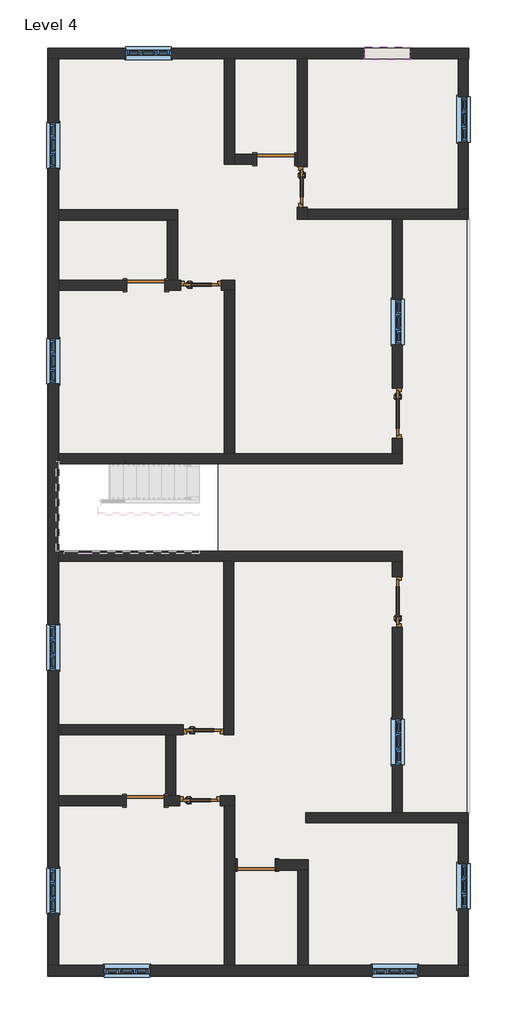
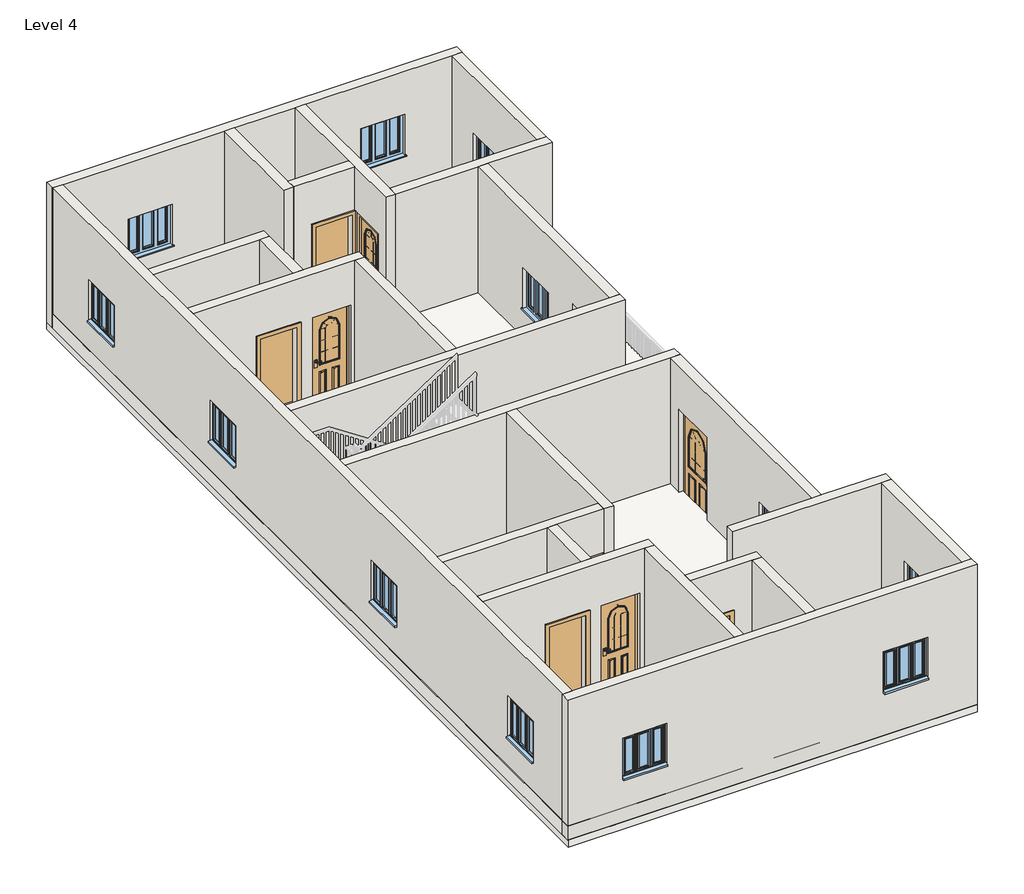
# One storey, part 1 of 3: 25 walls, 12 windows, 10 doors, 1 roof, 1 slab.
"""IFC4 building model written with IfcOpenShell, lengths in millimetres."""

from ifc_helpers import new_model, si_unit, frame, origin, place, context, project, spatial, polyline, outline, extrude, faceted_brep, transform, mapped, element, save
from components import doors_extsgl_w_glazing_bars_arched_1010x2110mm_bccdb1b2, doors_extsgl_w_glazing_bars_arched_1010x2110mm_5c897e1f, doors_extsgl_w_glazing_bars_arched_810x2110mm_57ea6d9e, doors_extsgl_w_glazing_bars_arched_810x2110mm_84a0a083, door_fadea3f2, windows_tpl_w_glazing_bars_910x910mm_9d987a72

model = new_model("IFC4")

# Units and contexts
model_context = context("Model", 3, world=origin())
ifc_project = project(units=[si_unit("LENGTHUNIT", "METRE", prefix="MILLI")], contexts=[model_context])

# Site, building, storey
site = spatial("IfcSite", under=ifc_project)
building = spatial("IfcBuilding", under=site)
storey = spatial("IfcBuildingStorey", under=building, Name="Level 4", Elevation=9144.0)

# Doors
placement = place(None, origin())
doors_extsgl_w_glazing_bars_arched_1010x2110mm_shape = doors_extsgl_w_glazing_bars_arched_1010x2110mm_bccdb1b2(model_context)
element("IfcDoor", 1, ObjectType="Doors_ExtSgl_w-Glazing_Bars_Arched : 1010x2110mm", at=placement, inside=storey, context=model_context, shape_type="MappedRepresentation", body=[
    mapped(doors_extsgl_w_glazing_bars_arched_1010x2110mm_shape, transform((1850.5605895, 2208.5797121, 9144.0), x_axis=(0.0, -1.0, 0.0), y_axis=(1.0, 0.0, 0.0), z_axis=(0.0, 0.0, 1.0))),
])
doors_extsgl_w_glazing_bars_arched_1010x2110mm_2_shape = doors_extsgl_w_glazing_bars_arched_1010x2110mm_5c897e1f(model_context)
element("IfcDoor", 2, ObjectType="Doors_ExtSgl_w-Glazing_Bars_Arched : 1010x2110mm", at=placement, inside=storey, context=model_context, shape_type="MappedRepresentation", body=[
    mapped(doors_extsgl_w_glazing_bars_arched_1010x2110mm_2_shape, transform((1850.5605895, -1576.0202879, 9144.0), x_axis=(0.0, 1.0, 0.0), y_axis=(-1.0, 0.0, 0.0), z_axis=(0.0, 0.0, 1.0))),
])
doors_extsgl_w_glazing_bars_arched_810x2110mm_shape = doors_extsgl_w_glazing_bars_arched_810x2110mm_57ea6d9e(model_context)
element("IfcDoor", 3, ObjectType="Doors_ExtSgl_w-Glazing_Bars_Arched : 810x2110mm", at=placement, inside=storey, context=model_context, shape_type="MappedRepresentation", body=[
    mapped(doors_extsgl_w_glazing_bars_arched_810x2110mm_shape, transform((-2086.4394105, 4773.9797121, 9144.0), x_axis=(1.0, 0.0, 0.0), y_axis=(0.0, 1.0, 0.0), z_axis=(0.0, 0.0, 1.0))),
])
element("IfcDoor", 4, ObjectType="Doors_ExtSgl_w-Glazing_Bars_Arched : 810x2110mm", at=placement, inside=storey, context=model_context, shape_type="MappedRepresentation", body=[
    mapped(doors_extsgl_w_glazing_bars_arched_810x2110mm_shape, transform((-2105.4894105, -5563.8202879, 9144.0), x_axis=(1.0, 0.0, 0.0), y_axis=(0.0, 1.0, 0.0), z_axis=(0.0, 0.0, 1.0))),
])
doors_extsgl_w_glazing_bars_arched_810x2110mm_2_shape = doors_extsgl_w_glazing_bars_arched_810x2110mm_84a0a083(model_context)
element("IfcDoor", 5, ObjectType="Doors_ExtSgl_w-Glazing_Bars_Arched : 810x2110mm", at=placement, inside=storey, context=model_context, shape_type="MappedRepresentation", body=[
    mapped(doors_extsgl_w_glazing_bars_arched_810x2110mm_2_shape, transform((-2035.6394105, -4141.4202879, 9144.0), x_axis=(1.0, 0.0, 0.0), y_axis=(0.0, 1.0, 0.0), z_axis=(0.0, 0.0, 1.0))),
])
element("IfcDoor", 6, ObjectType="Doors_ExtSgl_w-Glazing_Bars_Arched : 810x2110mm", at=placement, inside=storey, context=model_context, shape_type="MappedRepresentation", body=[
    mapped(doors_extsgl_w_glazing_bars_arched_810x2110mm_2_shape, transform((-54.4394105, 6748.5640518, 9144.0), x_axis=(0.0, -1.0, 0.0), y_axis=(1.0, 0.0, 0.0), z_axis=(0.0, 0.0, 1.0))),
])
door_shape = door_fadea3f2(model_context)
element("IfcDoor", 7, ObjectType="Single-Flush : 30\" x 80\"", at=placement, inside=storey, context=model_context, shape_type="MappedRepresentation", body=[
    mapped(door_shape, transform((-3204.0394105, -5563.8202879, 9144.0), x_axis=(1.0, 0.0, 0.0), y_axis=(0.0, 1.0, 0.0), z_axis=(0.0, 0.0, 1.0))),
])
element("IfcDoor", 8, ObjectType="Single-Flush : 30\" x 80\"", at=placement, inside=storey, context=model_context, shape_type="MappedRepresentation", body=[
    mapped(door_shape, transform((-981.5394105, -6850.9128362, 9144.0), x_axis=(-1.0, 0.0, 0.0), y_axis=(0.0, -1.0, 0.0), z_axis=(0.0, 0.0, 1.0))),
])
element("IfcDoor", 9, ObjectType="Single-Flush : 30\" x 80\"", at=placement, inside=storey, context=model_context, shape_type="MappedRepresentation", body=[
    mapped(door_shape, transform((-3191.3394105, 4773.9797121, 9144.0), x_axis=(1.0, 0.0, 0.0), y_axis=(0.0, 1.0, 0.0), z_axis=(0.0, 0.0, 1.0))),
])
element("IfcDoor", 10, ObjectType="Single-Flush : 30\" x 80\"", at=placement, inside=storey, context=model_context, shape_type="MappedRepresentation", body=[
    mapped(door_shape, transform((-587.8394105, 7301.2797121, 9144.0), x_axis=(1.0, 0.0, 0.0), y_axis=(0.0, 1.0, 0.0), z_axis=(0.0, 0.0, 1.0))),
])

# Roof
element("IfcRoof", 11, ObjectType="Generic - 12\"", at=placement, inside=storey, context=model_context, shape_type="SweptSolid", body=[
    extrude(outline(polyline([(3272.9605895, 9523.7797121), (3272.9605895, -9069.0202879), (-5159.8394105, -9069.0202879), (-5159.8394105, 9523.7797121), (3272.9605895, 9523.7797121)]), holes=[polyline([(-1756.1922756, 1192.5797121), (-4943.9394105, 1192.5797121), (-4943.9394105, -560.0202879), (-1756.1922756, -560.0202879), (-1756.1922756, 1192.5797121)])]), frame((0.0, 0.0, 9144.0), z_axis=(0.0, 0.0, 1.0), x_axis=(1.0, 0.0, 0.0)), (0.0, 0.0, 1.0), 304.8),
])

# Slab
element("IfcSlab", 12, ObjectType="Generic - 12\"", at=placement, inside=storey, context=model_context, shape_type="SweptSolid", body=[
    extrude(outline(polyline([(3272.9605895, 9523.7797121), (3272.9605895, -9081.7202879), (-5159.8394105, -9081.7202879), (-5159.8394105, 9523.7797121), (3272.9605895, 9523.7797121)]), holes=[polyline([(-1756.1922756, 1192.5797121), (-4943.9394105, 1192.5797121), (-4943.9394105, -560.0202879), (-1756.1922756, -560.0202879), (-1756.1922756, 1192.5797121)])]), frame((0.0, 0.0, 8991.6), z_axis=(0.0, 0.0, 1.0), x_axis=(1.0, 0.0, 0.0)), (0.0, 0.0, 1.0), 152.4),
])

# Walls
element("IfcWall", 13, ObjectType="Generic - 4.5\" p", at=placement, inside=storey, context=model_context, shape_type="Brep", body=[
    faceted_brep([(-2810.3394105, 4672.3797121, 11176.0), (-2810.3394105, 4672.3797121, 9144.0), (-2491.4394105, 4672.3797121, 9144.0), (-2491.4394105, 4672.3797121, 11254.0), (-1681.4394105, 4672.3797121, 11254.0), (-1681.4394105, 4672.3797121, 9144.0), (-1616.5394105, 4672.3797121, 9144.0), (-1413.3394105, 4672.3797121, 9144.0), (-1413.3394105, 4672.3797121, 12192.0), (-1616.5394105, 4672.3797121, 12192.0), (-4943.9394105, 4672.3797121, 12192.0), (-4943.9394105, 4672.3797121, 9144.0), (-3572.3394105, 4672.3797121, 9144.0), (-3572.3394105, 4672.3797121, 11176.0), (-2491.4394105, 4875.5797121, 9144.0), (-2556.3394105, 4875.5797121, 9144.0), (-2759.5394105, 4875.5797121, 9144.0), (-2810.3394105, 4875.5797121, 9144.0), (-2810.3394105, 4875.5797121, 11176.0), (-3572.3394105, 4875.5797121, 11176.0), (-3572.3394105, 4875.5797121, 9144.0), (-4943.9394105, 4875.5797121, 9144.0), (-4943.9394105, 4875.5797121, 12192.0), (-2759.5394105, 4875.5797121, 12192.0), (-2556.3394105, 4875.5797121, 12192.0), (-1413.3394105, 4875.5797121, 12192.0), (-1413.3394105, 4875.5797121, 9144.0), (-1681.4394105, 4875.5797121, 9144.0), (-1681.4394105, 4875.5797121, 11254.0), (-2491.4394105, 4875.5797121, 11254.0)], [[[0, 1, 2, 3, 4, 5, 6, 7, 8, 9, 10, 11, 12, 13]], [[14, 15, 16, 17, 18, 19, 20, 21, 22, 23, 24, 25, 26, 27, 28, 29]], [[7, 6, 5, 27, 26]], [[12, 11, 21, 20]], [[2, 1, 17, 16, 15, 14]], [[10, 9, 8, 25, 24, 23, 22]], [[11, 10, 22, 21]], [[8, 7, 26, 25]], [[14, 29, 3, 2]], [[28, 27, 5, 4]], [[29, 28, 4, 3]], [[18, 17, 1, 0]], [[19, 18, 0, 13]], [[20, 19, 13, 12]]]),
])
element("IfcWall", 14, ObjectType="Generic - 4.5\" p", at=placement, inside=storey, context=model_context, shape_type="SweptSolid", body=[
    extrude(outline(polyline([(-1616.5394105, 1395.7797121), (-1616.5394105, 4672.3797121), (-1413.3394105, 4672.3797121), (-1413.3394105, 1395.7797121), (-1616.5394105, 1395.7797121)])), frame((0.0, 0.0, 9144.0), z_axis=(0.0, 0.0, 1.0), x_axis=(1.0, 0.0, 0.0)), (0.0, 0.0, 1.0), 3048.0),
])
element("IfcWall", 15, ObjectType="Generic - 4.5\" p", at=placement, inside=storey, context=model_context, shape_type="Brep", body=[
    faceted_brep([(-4943.9394105, 6082.1542467, 9144.0), (-2759.5394105, 6082.1542467, 9144.0), (-2556.3394105, 6082.1542467, 9144.0), (-2556.3394105, 6082.1542467, 12192.0), (-2759.5394105, 6082.1542467, 12192.0), (-4943.9394105, 6082.1542467, 12192.0), (-4943.9394105, 6285.3542467, 9144.0), (-4943.9394105, 6285.3542467, 12192.0), (-2556.3394105, 6285.3542467, 12192.0), (-2556.3394105, 6285.3542467, 9144.0)], [[[0, 1, 2, 3, 4, 5]], [[6, 7, 8, 9]], [[2, 1, 0, 6, 9]], [[5, 4, 3, 8, 7]], [[0, 5, 7, 6]], [[3, 2, 9, 8]]]),
])
element("IfcWall", 16, ObjectType="Generic - 4.5\" p", at=placement, inside=storey, context=model_context, shape_type="SweptSolid", body=[
    extrude(outline(polyline([(-2759.5394105, 4875.5797121), (-2759.5394105, 6082.1542467), (-2556.3394105, 6082.1542467), (-2556.3394105, 4875.5797121), (-2759.5394105, 4875.5797121)])), frame((0.0, 0.0, 9144.0), z_axis=(0.0, 0.0, 1.0), x_axis=(1.0, 0.0, 0.0)), (0.0, 0.0, 1.0), 3048.0),
])
element("IfcWall", 17, ObjectType="Generic - 4.5\" p", at=placement, inside=storey, context=model_context, shape_type="Brep", body=[
    faceted_brep([(-1616.5394105, 9320.5797121, 9144.0), (-1616.5394105, 7199.6797121, 9144.0), (-1616.5394105, 7199.6797121, 12192.0), (-1616.5394105, 9320.5797121, 12192.0), (-1413.3394105, 9320.5797121, 9144.0), (-1413.3394105, 9320.5797121, 12192.0), (-1413.3394105, 7402.8797121, 12192.0), (-1413.3394105, 7199.6797121, 12192.0), (-1413.3394105, 7199.6797121, 9144.0), (-1413.3394105, 7402.8797121, 9144.0)], [[[0, 1, 2, 3]], [[4, 5, 6, 7, 8, 9]], [[1, 0, 4, 9, 8]], [[3, 2, 7, 6, 5]], [[0, 3, 5, 4]], [[2, 1, 8, 7]]]),
])
element("IfcWall", 18, ObjectType="Generic - 4.5\" p", at=placement, inside=storey, context=model_context, shape_type="SweptSolid", body=[
    extrude(outline(polyline([(11176.0, -206.8394105), (9144.0, -206.8394105), (9144.0, -156.0394105), (12192.0, -156.0394105), (12192.0, -1413.3394105), (9144.0, -1413.3394105), (9144.0, -968.8394105), (11176.0, -968.8394105), (11176.0, -206.8394105)])), frame((0.0, 7199.6797121, 0.0), z_axis=(0.0, 1.0, 0.0), x_axis=(0.0, 0.0, 1.0)), (0.0, 0.0, 1.0), 203.2),
])
element("IfcWall", 19, ObjectType="Generic - 4.5\" p", at=placement, inside=storey, context=model_context, shape_type="Brep", body=[
    faceted_brep([(-156.0394105, 6343.5640518, 11254.0), (-156.0394105, 6343.5640518, 9144.0), (-156.0394105, 6094.2483916, 9144.0), (-156.0394105, 6094.2483916, 12192.0), (-156.0394105, 7199.6797121, 12192.0), (-156.0394105, 7402.8797121, 12192.0), (-156.0394105, 9320.5797121, 12192.0), (-156.0394105, 9320.5797121, 9144.0), (-156.0394105, 7402.8797121, 9144.0), (-156.0394105, 7199.6797121, 9144.0), (-156.0394105, 7153.5640518, 9144.0), (-156.0394105, 7153.5640518, 11254.0), (47.1605895, 6094.2483916, 9144.0), (47.1605895, 6297.4483916, 9144.0), (47.1605895, 6343.5640518, 9144.0), (47.1605895, 6343.5640518, 11254.0), (47.1605895, 7153.5640518, 11254.0), (47.1605895, 7153.5640518, 9144.0), (47.1605895, 9320.5797121, 9144.0), (47.1605895, 9320.5797121, 12192.0), (47.1605895, 6297.4483916, 12192.0), (47.1605895, 6094.2483916, 12192.0)], [[[0, 1, 2, 3, 4, 5, 6, 7, 8, 9, 10, 11]], [[12, 13, 14, 15, 16, 17, 18, 19, 20, 21]], [[2, 1, 14, 13, 12]], [[10, 9, 8, 7, 18, 17]], [[6, 5, 4, 3, 21, 20, 19]], [[7, 6, 19, 18]], [[3, 2, 12, 21]], [[17, 16, 11, 10]], [[15, 14, 1, 0]], [[16, 15, 0, 11]]]),
])
element("IfcWall", 20, ObjectType="Generic - 4.5\" p", at=placement, inside=storey, context=model_context, shape_type="Brep", body=[
    faceted_brep([(47.1605895, 6094.2483916, 9144.0), (1748.9605895, 6094.2483916, 9144.0), (1952.1605895, 6094.2483916, 9144.0), (3272.9605895, 6094.2483916, 9144.0), (3272.9605895, 6094.2483916, 12192.0), (1952.1605895, 6094.2483916, 12192.0), (1748.9605895, 6094.2483916, 12192.0), (47.1605895, 6094.2483916, 12192.0), (47.1605895, 6297.4483916, 9144.0), (47.1605895, 6297.4483916, 12192.0), (3069.7605895, 6297.4483916, 12192.0), (3272.9605895, 6297.4483916, 12192.0), (3272.9605895, 6297.4483916, 9144.0), (3069.7605895, 6297.4483916, 9144.0)], [[[0, 1, 2, 3, 4, 5, 6, 7]], [[8, 9, 10, 11, 12, 13]], [[3, 2, 1, 0, 8, 13, 12]], [[7, 6, 5, 4, 11, 10, 9]], [[0, 7, 9, 8]], [[4, 3, 12, 11]]]),
])
element("IfcWall", 21, ObjectType="Generic - 4.5\" p", at=placement, inside=storey, context=model_context, shape_type="Brep", body=[
    faceted_brep([(-4943.9394105, 1192.5797121, 9144.0), (1952.1605895, 1192.5797121, 9144.0), (1952.1605895, 1192.5797121, 12192.0), (-4943.9394105, 1192.5797121, 12192.0), (-4943.9394105, 1395.7797121, 9144.0), (-4943.9394105, 1395.7797121, 12192.0), (-1616.5394105, 1395.7797121, 12192.0), (-1413.3394105, 1395.7797121, 12192.0), (1748.9605895, 1395.7797121, 12192.0), (1952.1605895, 1395.7797121, 12192.0), (1952.1605895, 1395.7797121, 9144.0), (1748.9605895, 1395.7797121, 9144.0), (-1413.3394105, 1395.7797121, 9144.0), (-1616.5394105, 1395.7797121, 9144.0)], [[[0, 1, 2, 3]], [[4, 5, 6, 7, 8, 9, 10, 11, 12, 13]], [[1, 0, 4, 13, 12, 11, 10]], [[3, 2, 9, 8, 7, 6, 5]], [[0, 3, 5, 4]], [[2, 1, 10, 9]]]),
])
element("IfcWall", 22, ObjectType="Generic - 4.5\" p", at=placement, inside=storey, context=model_context, shape_type="Brep", body=[
    faceted_brep([(-4943.9394105, -763.2202879, 9144.0), (-1629.2394105, -763.2202879, 9144.0), (-1426.0394105, -763.2202879, 9144.0), (1748.9605895, -763.2202879, 9144.0), (1952.1605895, -763.2202879, 9144.0), (1952.1605895, -763.2202879, 12192.0), (1748.9605895, -763.2202879, 12192.0), (-1426.0394105, -763.2202879, 12192.0), (-1629.2394105, -763.2202879, 12192.0), (-4943.9394105, -763.2202879, 12192.0), (-4943.9394105, -560.0202879, 9144.0), (-4943.9394105, -560.0202879, 12192.0), (1952.1605895, -560.0202879, 12192.0), (1952.1605895, -560.0202879, 9144.0)], [[[0, 1, 2, 3, 4, 5, 6, 7, 8, 9]], [[10, 11, 12, 13]], [[4, 3, 2, 1, 0, 10, 13]], [[9, 8, 7, 6, 5, 12, 11]], [[0, 9, 11, 10]], [[5, 4, 13, 12]]]),
])
element("IfcWall", 23, ObjectType="Generic - 4.5\" p", at=placement, inside=storey, context=model_context, shape_type="Brep", body=[
    faceted_brep([(-1629.2394105, -763.2202879, 9144.0), (-1629.2394105, -4039.8202879, 9144.0), (-1629.2394105, -4243.0202879, 9144.0), (-1629.2394105, -4243.0202879, 12192.0), (-1629.2394105, -4039.8202879, 12192.0), (-1629.2394105, -763.2202879, 12192.0), (-1426.0394105, -763.2202879, 9144.0), (-1426.0394105, -763.2202879, 12192.0), (-1426.0394105, -4243.0202879, 12192.0), (-1426.0394105, -4243.0202879, 9144.0)], [[[0, 1, 2, 3, 4, 5]], [[6, 7, 8, 9]], [[2, 1, 0, 6, 9]], [[5, 4, 3, 8, 7]], [[0, 5, 7, 6]], [[3, 2, 9, 8]]]),
])
element("IfcWall", 24, ObjectType="Generic - 4.5\" p", at=placement, inside=storey, context=model_context, shape_type="Brep", body=[
    faceted_brep([(-1630.6394105, -4243.0202879, 11254.0), (-1630.6394105, -4243.0202879, 9144.0), (-1629.2394105, -4243.0202879, 9144.0), (-1629.2394105, -4243.0202879, 12192.0), (-2594.4394105, -4243.0202879, 12192.0), (-2797.6394105, -4243.0202879, 12192.0), (-4943.9394105, -4243.0202879, 12192.0), (-4943.9394105, -4243.0202879, 9144.0), (-2797.6394105, -4243.0202879, 9144.0), (-2594.4394105, -4243.0202879, 9144.0), (-2440.6394105, -4243.0202879, 9144.0), (-2440.6394105, -4243.0202879, 11254.0), (-1629.2394105, -4039.8202879, 9144.0), (-1630.6394105, -4039.8202879, 9144.0), (-1630.6394105, -4039.8202879, 11254.0), (-2440.6394105, -4039.8202879, 11254.0), (-2440.6394105, -4039.8202879, 9144.0), (-4943.9394105, -4039.8202879, 9144.0), (-4943.9394105, -4039.8202879, 12192.0), (-1629.2394105, -4039.8202879, 12192.0)], [[[0, 1, 2, 3, 4, 5, 6, 7, 8, 9, 10, 11]], [[12, 13, 14, 15, 16, 17, 18, 19]], [[2, 1, 13, 12]], [[10, 9, 8, 7, 17, 16]], [[6, 5, 4, 3, 19, 18]], [[3, 2, 12, 19]], [[7, 6, 18, 17]], [[16, 15, 11, 10]], [[14, 13, 1, 0]], [[15, 14, 0, 11]]]),
])
element("IfcWall", 25, ObjectType="Generic - 4.5\" p", at=placement, inside=storey, context=model_context, shape_type="Brep", body=[
    faceted_brep([(-2823.0394105, -5665.4202879, 11176.0), (-2823.0394105, -5665.4202879, 9144.0), (-2510.4894105, -5665.4202879, 9144.0), (-2510.4894105, -5665.4202879, 11254.0), (-1700.4894105, -5665.4202879, 11254.0), (-1700.4894105, -5665.4202879, 9144.0), (-1616.5394105, -5665.4202879, 9144.0), (-1413.3394105, -5665.4202879, 9144.0), (-1413.3394105, -5665.4202879, 12192.0), (-1616.5394105, -5665.4202879, 12192.0), (-4943.9394105, -5665.4202879, 12192.0), (-4943.9394105, -5665.4202879, 9144.0), (-3585.0394105, -5665.4202879, 9144.0), (-3585.0394105, -5665.4202879, 11176.0), (-2510.4894105, -5462.2202879, 9144.0), (-2594.4394105, -5462.2202879, 9144.0), (-2797.6394105, -5462.2202879, 9144.0), (-2823.0394105, -5462.2202879, 9144.0), (-2823.0394105, -5462.2202879, 11176.0), (-3585.0394105, -5462.2202879, 11176.0), (-3585.0394105, -5462.2202879, 9144.0), (-4943.9394105, -5462.2202879, 9144.0), (-4943.9394105, -5462.2202879, 12192.0), (-2797.6394105, -5462.2202879, 12192.0), (-2594.4394105, -5462.2202879, 12192.0), (-1413.3394105, -5462.2202879, 12192.0), (-1413.3394105, -5462.2202879, 9144.0), (-1700.4894105, -5462.2202879, 9144.0), (-1700.4894105, -5462.2202879, 11254.0), (-2510.4894105, -5462.2202879, 11254.0)], [[[0, 1, 2, 3, 4, 5, 6, 7, 8, 9, 10, 11, 12, 13]], [[14, 15, 16, 17, 18, 19, 20, 21, 22, 23, 24, 25, 26, 27, 28, 29]], [[7, 6, 5, 27, 26]], [[12, 11, 21, 20]], [[2, 1, 17, 16, 15, 14]], [[10, 9, 8, 25, 24, 23, 22]], [[11, 10, 22, 21]], [[8, 7, 26, 25]], [[14, 29, 3, 2]], [[28, 27, 5, 4]], [[29, 28, 4, 3]], [[18, 17, 1, 0]], [[19, 18, 0, 13]], [[20, 19, 13, 12]]]),
])
element("IfcWall", 26, ObjectType="Generic - 4.5\" p", at=placement, inside=storey, context=model_context, shape_type="SweptSolid", body=[
    extrude(outline(polyline([(-2797.6394105, -5462.2202879), (-2797.6394105, -4243.0202879), (-2594.4394105, -4243.0202879), (-2594.4394105, -5462.2202879), (-2797.6394105, -5462.2202879)])), frame((0.0, 0.0, 9144.0), z_axis=(0.0, 0.0, 1.0), x_axis=(1.0, 0.0, 0.0)), (0.0, 0.0, 1.0), 3048.0),
])
element("IfcWall", 27, ObjectType="Generic - 4.5\" p", at=placement, inside=storey, context=model_context, shape_type="Brep", body=[
    faceted_brep([(-1616.5394105, -5665.4202879, 9144.0), (-1616.5394105, -8865.8202879, 9144.0), (-1616.5394105, -8865.8202879, 12192.0), (-1616.5394105, -5665.4202879, 12192.0), (-1413.3394105, -5665.4202879, 9144.0), (-1413.3394105, -5665.4202879, 12192.0), (-1413.3394105, -6749.3128362, 12192.0), (-1413.3394105, -6952.5128362, 12192.0), (-1413.3394105, -8865.8202879, 12192.0), (-1413.3394105, -8865.8202879, 9144.0), (-1413.3394105, -6952.5128362, 9144.0), (-1413.3394105, -6749.3128362, 9144.0)], [[[0, 1, 2, 3]], [[4, 5, 6, 7, 8, 9, 10, 11]], [[1, 0, 4, 11, 10, 9]], [[3, 2, 8, 7, 6, 5]], [[0, 3, 5, 4]], [[2, 1, 9, 8]]]),
])
element("IfcWall", 28, ObjectType="Generic - 4.5\" p", at=placement, inside=storey, context=model_context, shape_type="Brep", body=[
    faceted_brep([(-1413.3394105, -6952.5128362, 9144.0), (-1362.5394105, -6952.5128362, 9144.0), (-1362.5394105, -6952.5128362, 11176.0), (-600.5394105, -6952.5128362, 11176.0), (-600.5394105, -6952.5128362, 9144.0), (-143.3394105, -6952.5128362, 9144.0), (59.8605895, -6952.5128362, 9144.0), (59.8605895, -6952.5128362, 12192.0), (-143.3394105, -6952.5128362, 12192.0), (-1413.3394105, -6952.5128362, 12192.0), (-1362.5394105, -6749.3128362, 11176.0), (-1362.5394105, -6749.3128362, 9144.0), (-1413.3394105, -6749.3128362, 9144.0), (-1413.3394105, -6749.3128362, 12192.0), (59.8605895, -6749.3128362, 12192.0), (59.8605895, -6749.3128362, 9144.0), (-600.5394105, -6749.3128362, 9144.0), (-600.5394105, -6749.3128362, 11176.0)], [[[0, 1, 2, 3, 4, 5, 6, 7, 8, 9]], [[10, 11, 12, 13, 14, 15, 16, 17]], [[16, 15, 6, 5, 4]], [[12, 11, 1, 0]], [[9, 8, 7, 14, 13]], [[0, 9, 13, 12]], [[7, 6, 15, 14]], [[2, 1, 11, 10]], [[3, 2, 10, 17]], [[4, 3, 17, 16]]]),
])
element("IfcWall", 29, ObjectType="Generic - 4.5\" p", at=placement, inside=storey, context=model_context, shape_type="SweptSolid", body=[
    extrude(outline(polyline([(-143.3394105, -8865.8202879), (-143.3394105, -6952.5128362), (59.8605895, -6952.5128362), (59.8605895, -8865.8202879), (-143.3394105, -8865.8202879)])), frame((0.0, 0.0, 9144.0), z_axis=(0.0, 0.0, 1.0), x_axis=(1.0, 0.0, 0.0)), (0.0, 0.0, 1.0), 3048.0),
])
element("IfcWall", 30, ObjectType="Generic - 4.5\" p", at=placement, inside=storey, context=model_context, shape_type="Brep", body=[
    faceted_brep([(3272.9605895, -5805.1202879, 9144.0), (1952.1605895, -5805.1202879, 9144.0), (1748.9605895, -5805.1202879, 9144.0), (9.0605895, -5805.1202879, 9144.0), (9.0605895, -5805.1202879, 12192.0), (1748.9605895, -5805.1202879, 12192.0), (1952.1605895, -5805.1202879, 12192.0), (3272.9605895, -5805.1202879, 12192.0), (3272.9605895, -6008.3202879, 9144.0), (3272.9605895, -6008.3202879, 12192.0), (3069.7605895, -6008.3202879, 12192.0), (9.0605895, -6008.3202879, 12192.0), (9.0605895, -6008.3202879, 9144.0), (3069.7605895, -6008.3202879, 9144.0)], [[[0, 1, 2, 3, 4, 5, 6, 7]], [[8, 9, 10, 11, 12, 13]], [[3, 2, 1, 0, 8, 13, 12]], [[4, 3, 12, 11]], [[7, 6, 5, 4, 11, 10, 9]], [[0, 7, 9, 8]]]),
])
element("IfcWall", 31, ObjectType="Generic - 9\" w", at=placement, inside=storey, context=model_context, shape_type="Brep", body=[
    faceted_brep([(-5159.8394105, 9320.5797121, 9144.0), (-5147.1394105, 9320.5797121, 9144.0), (-4943.9394105, 9320.5797121, 9144.0), (-1616.5394105, 9320.5797121, 9144.0), (-1413.3394105, 9320.5797121, 9144.0), (-156.0394105, 9320.5797121, 9144.0), (47.1605895, 9320.5797121, 9144.0), (3069.7605895, 9320.5797121, 9144.0), (3272.9605895, 9320.5797121, 9144.0), (3285.6605895, 9320.5797121, 9144.0), (3285.6605895, 9320.5797121, 12192.0), (3272.9605895, 9320.5797121, 12192.0), (3069.7605895, 9320.5797121, 12192.0), (47.1605895, 9320.5797121, 12192.0), (-156.0394105, 9320.5797121, 12192.0), (-1413.3394105, 9320.5797121, 12192.0), (-1616.5394105, 9320.5797121, 12192.0), (-4943.9394105, 9320.5797121, 12192.0), (-5147.1394105, 9320.5797121, 12192.0), (-5159.8394105, 9320.5797121, 12192.0), (1192.3605895, 9320.5797121, 11254.0), (2102.3605895, 9320.5797121, 11254.0), (2102.3605895, 9320.5797121, 10344.0), (1192.3605895, 9320.5797121, 10344.0), (-3595.5394105, 9320.5797121, 10968.4), (-2685.5394105, 9320.5797121, 10968.4), (-2685.5394105, 9320.5797121, 10058.4), (-3595.5394105, 9320.5797121, 10058.4), (-5159.8394105, 9523.7797121, 9144.0), (-5159.8394105, 9523.7797121, 12192.0), (3285.6605895, 9523.7797121, 12192.0), (3285.6605895, 9523.7797121, 9144.0), (1192.3605895, 9523.7797121, 11254.0), (1192.3605895, 9523.7797121, 10344.0), (2102.3605895, 9523.7797121, 10344.0), (2102.3605895, 9523.7797121, 11254.0), (-3595.5394105, 9523.7797121, 10968.4), (-3595.5394105, 9523.7797121, 10058.4), (-2685.5394105, 9523.7797121, 10058.4), (-2685.5394105, 9523.7797121, 10968.4)], [[[0, 1, 2, 3, 4, 5, 6, 7, 8, 9, 10, 11, 12, 13, 14, 15, 16, 17, 18, 19], [20, 21, 22, 23], [24, 25, 26, 27]], [[28, 29, 30, 31], [32, 33, 34, 35], [36, 37, 38, 39]], [[9, 8, 7, 6, 5, 4, 3, 2, 1, 0, 28, 31]], [[10, 9, 31, 30]], [[19, 18, 17, 16, 15, 14, 13, 12, 11, 10, 30, 29]], [[0, 19, 29, 28]], [[33, 32, 20, 23]], [[34, 33, 23, 22]], [[35, 34, 22, 21]], [[32, 35, 21, 20]], [[37, 36, 24, 27]], [[38, 37, 27, 26]], [[39, 38, 26, 25]], [[36, 39, 25, 24]]]),
])
element("IfcWall", 32, ObjectType="Generic - 9\" w", at=placement, inside=storey, context=model_context, shape_type="Brep", body=[
    faceted_brep([(3272.9605895, -8865.8202879, 9144.0), (3069.7605895, -8865.8202879, 9144.0), (59.8605895, -8865.8202879, 9144.0), (-143.3394105, -8865.8202879, 9144.0), (-1413.3394105, -8865.8202879, 9144.0), (-1616.5394105, -8865.8202879, 9144.0), (-4943.9394105, -8865.8202879, 9144.0), (-5147.1394105, -8865.8202879, 9144.0), (-5159.8394105, -8865.8202879, 9144.0), (-5159.8394105, -8865.8202879, 12192.0), (-5147.1394105, -8865.8202879, 12192.0), (-4943.9394105, -8865.8202879, 12192.0), (-1616.5394105, -8865.8202879, 12192.0), (-1413.3394105, -8865.8202879, 12192.0), (-143.3394105, -8865.8202879, 12192.0), (59.8605895, -8865.8202879, 12192.0), (3069.7605895, -8865.8202879, 12192.0), (3272.9605895, -8865.8202879, 12192.0), (-3117.3394105, -8865.8202879, 10968.4), (-4027.3394105, -8865.8202879, 10968.4), (-4027.3394105, -8865.8202879, 10058.4), (-3117.3394105, -8865.8202879, 10058.4), (2254.7605895, -8865.8202879, 10968.4), (1344.7605895, -8865.8202879, 10968.4), (1344.7605895, -8865.8202879, 10058.4), (2254.7605895, -8865.8202879, 10058.4), (3272.9605895, -9069.0202879, 9144.0), (3272.9605895, -9069.0202879, 12192.0), (-5159.8394105, -9069.0202879, 12192.0), (-5159.8394105, -9069.0202879, 9144.0), (-3117.3394105, -9069.0202879, 10968.4), (-3117.3394105, -9069.0202879, 10058.4), (-4027.3394105, -9069.0202879, 10058.4), (-4027.3394105, -9069.0202879, 10968.4), (2254.7605895, -9069.0202879, 10968.4), (2254.7605895, -9069.0202879, 10058.4), (1344.7605895, -9069.0202879, 10058.4), (1344.7605895, -9069.0202879, 10968.4)], [[[0, 1, 2, 3, 4, 5, 6, 7, 8, 9, 10, 11, 12, 13, 14, 15, 16, 17], [18, 19, 20, 21], [22, 23, 24, 25]], [[26, 27, 28, 29], [30, 31, 32, 33], [34, 35, 36, 37]], [[8, 7, 6, 5, 4, 3, 2, 1, 0, 26, 29]], [[9, 8, 29, 28]], [[17, 16, 15, 14, 13, 12, 11, 10, 9, 28, 27]], [[0, 17, 27, 26]], [[31, 30, 18, 21]], [[32, 31, 21, 20]], [[33, 32, 20, 19]], [[30, 33, 19, 18]], [[35, 34, 22, 25]], [[36, 35, 25, 24]], [[37, 36, 24, 23]], [[34, 37, 23, 22]]]),
])
element("IfcWall", 33, ObjectType="Generic - 9\" w", at=placement, inside=storey, context=model_context, shape_type="Brep", body=[
    faceted_brep([(-4943.9394105, -8865.8202879, 9144.0), (-4943.9394105, -5665.4202879, 9144.0), (-4943.9394105, -5462.2202879, 9144.0), (-4943.9394105, -4243.0202879, 9144.0), (-4943.9394105, -4039.8202879, 9144.0), (-4943.9394105, -763.2202879, 9144.0), (-4943.9394105, -560.0202879, 9144.0), (-4943.9394105, 1192.5797121, 9144.0), (-4943.9394105, 1395.7797121, 9144.0), (-4943.9394105, 4672.3797121, 9144.0), (-4943.9394105, 4875.5797121, 9144.0), (-4943.9394105, 6082.1542467, 9144.0), (-4943.9394105, 6285.3542467, 9144.0), (-4943.9394105, 9320.5797121, 9144.0), (-4943.9394105, 9320.5797121, 12192.0), (-4943.9394105, 6285.3542467, 12192.0), (-4943.9394105, 6082.1542467, 12192.0), (-4943.9394105, 4875.5797121, 12192.0), (-4943.9394105, 4672.3797121, 12192.0), (-4943.9394105, 1395.7797121, 12192.0), (-4943.9394105, 1192.5797121, 12192.0), (-4943.9394105, -560.0202879, 12192.0), (-4943.9394105, -763.2202879, 12192.0), (-4943.9394105, -4039.8202879, 12192.0), (-4943.9394105, -4243.0202879, 12192.0), (-4943.9394105, -5462.2202879, 12192.0), (-4943.9394105, -5665.4202879, 12192.0), (-4943.9394105, -8865.8202879, 12192.0), (-4943.9394105, -7822.2202879, 10968.4), (-4943.9394105, -6912.2202879, 10968.4), (-4943.9394105, -6912.2202879, 10058.4), (-4943.9394105, -7822.2202879, 10058.4), (-4943.9394105, -2945.4202879, 10968.4), (-4943.9394105, -2035.4202879, 10968.4), (-4943.9394105, -2035.4202879, 10058.4), (-4943.9394105, -2945.4202879, 10058.4), (-4943.9394105, 2794.9797121, 10968.4), (-4943.9394105, 3704.9797121, 10968.4), (-4943.9394105, 3704.9797121, 10058.4), (-4943.9394105, 2794.9797121, 10058.4), (-4943.9394105, 7125.7542467, 10968.4), (-4943.9394105, 8035.7542467, 10968.4), (-4943.9394105, 8035.7542467, 10058.4), (-4943.9394105, 7125.7542467, 10058.4), (-5147.1394105, -8865.8202879, 9144.0), (-5147.1394105, -8865.8202879, 12192.0), (-5147.1394105, 9320.5797121, 12192.0), (-5147.1394105, 9320.5797121, 9144.0), (-5147.1394105, -7822.2202879, 10968.4), (-5147.1394105, -7822.2202879, 10058.4), (-5147.1394105, -6912.2202879, 10058.4), (-5147.1394105, -6912.2202879, 10968.4), (-5147.1394105, -2945.4202879, 10968.4), (-5147.1394105, -2945.4202879, 10058.4), (-5147.1394105, -2035.4202879, 10058.4), (-5147.1394105, -2035.4202879, 10968.4), (-5147.1394105, 2794.9797121, 10968.4), (-5147.1394105, 2794.9797121, 10058.4), (-5147.1394105, 3704.9797121, 10058.4), (-5147.1394105, 3704.9797121, 10968.4), (-5147.1394105, 7125.7542467, 10968.4), (-5147.1394105, 7125.7542467, 10058.4), (-5147.1394105, 8035.7542467, 10058.4), (-5147.1394105, 8035.7542467, 10968.4)], [[[0, 1, 2, 3, 4, 5, 6, 7, 8, 9, 10, 11, 12, 13, 14, 15, 16, 17, 18, 19, 20, 21, 22, 23, 24, 25, 26, 27], [28, 29, 30, 31], [32, 33, 34, 35], [36, 37, 38, 39], [40, 41, 42, 43]], [[44, 45, 46, 47], [48, 49, 50, 51], [52, 53, 54, 55], [56, 57, 58, 59], [60, 61, 62, 63]], [[13, 12, 11, 10, 9, 8, 7, 6, 5, 4, 3, 2, 1, 0, 44, 47]], [[27, 26, 25, 24, 23, 22, 21, 20, 19, 18, 17, 16, 15, 14, 46, 45]], [[14, 13, 47, 46]], [[0, 27, 45, 44]], [[49, 48, 28, 31]], [[50, 49, 31, 30]], [[51, 50, 30, 29]], [[48, 51, 29, 28]], [[53, 52, 32, 35]], [[54, 53, 35, 34]], [[55, 54, 34, 33]], [[52, 55, 33, 32]], [[57, 56, 36, 39]], [[58, 57, 39, 38]], [[59, 58, 38, 37]], [[56, 59, 37, 36]], [[61, 60, 40, 43]], [[62, 61, 43, 42]], [[63, 62, 42, 41]], [[60, 63, 41, 40]]]),
])
element("IfcWall", 34, ObjectType="Generic - 9\" w", at=placement, inside=storey, context=model_context, shape_type="SweptSolid", body=[
    extrude(outline(polyline([(-8865.8202879, 9144.0), (-8865.8202879, 12192.0), (-6008.3202879, 12192.0), (-6008.3202879, 9144.0), (-8865.8202879, 9144.0)]), holes=[polyline([(-6823.3202879, 10968.4), (-7733.3202879, 10968.4), (-7733.3202879, 10058.4), (-6823.3202879, 10058.4), (-6823.3202879, 10968.4)])]), frame((3069.7605895, 0.0, 0.0), z_axis=(1.0, 0.0, 0.0), x_axis=(0.0, 1.0, 0.0)), (0.0, 0.0, 1.0), 203.2),
])
element("IfcWall", 35, ObjectType="Generic - 9\" w", at=placement, inside=storey, context=model_context, shape_type="SweptSolid", body=[
    extrude(outline(polyline([(9320.5797121, 9144.0), (6297.4483916, 9144.0), (6297.4483916, 12192.0), (9320.5797121, 12192.0), (9320.5797121, 9144.0)]), holes=[polyline([(8556.3797121, 10968.4), (7646.3797121, 10968.4), (7646.3797121, 10058.4), (8556.3797121, 10058.4), (8556.3797121, 10968.4)])]), frame((3069.7605895, 0.0, 0.0), z_axis=(1.0, 0.0, 0.0), x_axis=(0.0, 1.0, 0.0)), (0.0, 0.0, 1.0), 203.2),
])
element("IfcWall", 36, ObjectType="Generic - 9\" w", at=placement, inside=storey, context=model_context, shape_type="SweptSolid", body=[
    extrude(outline(polyline([(-763.2202879, 9144.0), (-1071.0202879, 9144.0), (-1071.0202879, 11254.0), (-2081.0202879, 11254.0), (-2081.0202879, 9144.0), (-5805.1202879, 9144.0), (-5805.1202879, 12192.0), (-763.2202879, 12192.0), (-763.2202879, 9144.0)]), holes=[polyline([(-3927.7202879, 10968.4), (-4837.7202879, 10968.4), (-4837.7202879, 10058.4), (-3927.7202879, 10058.4), (-3927.7202879, 10968.4)])]), frame((1748.9605895, 0.0, 0.0), z_axis=(1.0, 0.0, 0.0), x_axis=(0.0, 1.0, 0.0)), (0.0, 0.0, 1.0), 203.2),
])
element("IfcWall", 37, ObjectType="Generic - 9\" w", at=placement, inside=storey, context=model_context, shape_type="SweptSolid", body=[
    extrude(outline(polyline([(1703.5797121, 11254.0), (1703.5797121, 9144.0), (1395.7797121, 9144.0), (1395.7797121, 12192.0), (6094.2483916, 12192.0), (6094.2483916, 9144.0), (2713.5797121, 9144.0), (2713.5797121, 11254.0), (1703.5797121, 11254.0)]), holes=[polyline([(4492.3797121, 10968.4), (3582.3797121, 10968.4), (3582.3797121, 10058.4), (4492.3797121, 10058.4), (4492.3797121, 10968.4)])]), frame((1748.9605895, 0.0, 0.0), z_axis=(1.0, 0.0, 0.0), x_axis=(0.0, 1.0, 0.0)), (0.0, 0.0, 1.0), 203.2),
])

# Windows
windows_tpl_w_glazing_bars_910x910mm_shape = windows_tpl_w_glazing_bars_910x910mm_9d987a72(model_context)
element("IfcWindow", 38, ObjectType="Windows_Tpl_w-Glazing_Bars : 910x910mm", at=placement, inside=storey, context=model_context, shape_type="MappedRepresentation", body=[
    mapped(windows_tpl_w_glazing_bars_910x910mm_shape, transform((-3809.0060772, -8958.9637201, 8858.4), x_axis=(-1.0, 0.0, 0.0), y_axis=(0.0, -1.0, 0.0), z_axis=(0.0, 0.0, 1.0))),
])
element("IfcWindow", 39, ObjectType="Windows_Tpl_w-Glazing_Bars : 910x910mm", at=placement, inside=storey, context=model_context, shape_type="MappedRepresentation", body=[
    mapped(windows_tpl_w_glazing_bars_910x910mm_shape, transform((-5037.0828427, -7130.5536213, 8858.4), x_axis=(0.0, 1.0, 0.0), y_axis=(-1.0, 0.0, 0.0), z_axis=(0.0, 0.0, 1.0))),
])
element("IfcWindow", 40, ObjectType="Windows_Tpl_w-Glazing_Bars : 910x910mm", at=placement, inside=storey, context=model_context, shape_type="MappedRepresentation", body=[
    mapped(windows_tpl_w_glazing_bars_910x910mm_shape, transform((-5037.0828427, -2253.7536213, 8858.4), x_axis=(0.0, 1.0, 0.0), y_axis=(-1.0, 0.0, 0.0), z_axis=(0.0, 0.0, 1.0))),
])
element("IfcWindow", 41, ObjectType="Windows_Tpl_w-Glazing_Bars : 910x910mm", at=placement, inside=storey, context=model_context, shape_type="MappedRepresentation", body=[
    mapped(windows_tpl_w_glazing_bars_910x910mm_shape, transform((-5037.0828427, 3486.6463787, 8858.4), x_axis=(0.0, 1.0, 0.0), y_axis=(-1.0, 0.0, 0.0), z_axis=(0.0, 0.0, 1.0))),
])
element("IfcWindow", 42, ObjectType="Windows_Tpl_w-Glazing_Bars : 910x910mm", at=placement, inside=storey, context=model_context, shape_type="MappedRepresentation", body=[
    mapped(windows_tpl_w_glazing_bars_910x910mm_shape, transform((3162.9040216, 7864.7130454, 8858.4), x_axis=(0.0, -1.0, 0.0), y_axis=(1.0, 0.0, 0.0), z_axis=(0.0, 0.0, 1.0))),
])
element("IfcWindow", 43, ObjectType="Windows_Tpl_w-Glazing_Bars : 910x910mm", at=placement, inside=storey, context=model_context, shape_type="MappedRepresentation", body=[
    mapped(windows_tpl_w_glazing_bars_910x910mm_shape, transform((1884.0272561, 9413.7231443, 9144.0), x_axis=(1.0, 0.0, 0.0), y_axis=(0.0, 1.0, 0.0), z_axis=(0.0, 0.0, 1.0))),
])
element("IfcWindow", 44, ObjectType="Windows_Tpl_w-Glazing_Bars : 910x910mm", at=placement, inside=storey, context=model_context, shape_type="MappedRepresentation", body=[
    mapped(windows_tpl_w_glazing_bars_910x910mm_shape, transform((1563.0939228, -8958.9637201, 8858.4), x_axis=(-1.0, 0.0, 0.0), y_axis=(0.0, -1.0, 0.0), z_axis=(0.0, 0.0, 1.0))),
])
element("IfcWindow", 45, ObjectType="Windows_Tpl_w-Glazing_Bars : 910x910mm", at=placement, inside=storey, context=model_context, shape_type="MappedRepresentation", body=[
    mapped(windows_tpl_w_glazing_bars_910x910mm_shape, transform((3162.9040216, -7514.9869546, 8858.4), x_axis=(0.0, -1.0, 0.0), y_axis=(1.0, 0.0, 0.0), z_axis=(0.0, 0.0, 1.0))),
])
element("IfcWindow", 46, ObjectType="Windows_Tpl_w-Glazing_Bars : 910x910mm", at=placement, inside=storey, context=model_context, shape_type="MappedRepresentation", body=[
    mapped(windows_tpl_w_glazing_bars_910x910mm_shape, transform((-5037.0828427, 7817.4209133, 8858.4), x_axis=(0.0, 1.0, 0.0), y_axis=(-1.0, 0.0, 0.0), z_axis=(0.0, 0.0, 1.0))),
])
element("IfcWindow", 47, ObjectType="Windows_Tpl_w-Glazing_Bars : 910x910mm", at=placement, inside=storey, context=model_context, shape_type="MappedRepresentation", body=[
    mapped(windows_tpl_w_glazing_bars_910x910mm_shape, transform((-2903.8727439, 9413.7231443, 8858.4), x_axis=(1.0, 0.0, 0.0), y_axis=(0.0, 1.0, 0.0), z_axis=(0.0, 0.0, 1.0))),
])
element("IfcWindow", 48, ObjectType="Windows_Tpl_w-Glazing_Bars : 910x910mm", at=placement, inside=storey, context=model_context, shape_type="MappedRepresentation", body=[
    mapped(windows_tpl_w_glazing_bars_910x910mm_shape, transform((1842.1040216, -4619.3869546, 8858.4), x_axis=(0.0, -1.0, 0.0), y_axis=(1.0, 0.0, 0.0), z_axis=(0.0, 0.0, 1.0))),
])
element("IfcWindow", 49, ObjectType="Windows_Tpl_w-Glazing_Bars : 910x910mm", at=placement, inside=storey, context=model_context, shape_type="MappedRepresentation", body=[
    mapped(windows_tpl_w_glazing_bars_910x910mm_shape, transform((1842.1040216, 3800.7130454, 8858.4), x_axis=(0.0, -1.0, 0.0), y_axis=(1.0, 0.0, 0.0), z_axis=(0.0, 0.0, 1.0))),
])

save(model, "model.ifc")

# Revit data of these elements
# Type "Doors_ExtSgl_w-Glazing_Bars_Arched : 1010x2110mm"
#   Type Mark = "10"
#   Type Comments = "External Single"
#   Operation = "SingleSwingRight"
#   Construction Type Id = "SGL"
#   Keynote = "L20"
#   Analytic Construction = "Large single-glazed windows"
#   Wrap Layers (Int) from Ext = 177.5 mm
#   Wrap Layers (Ext) from Ext = 102.5 mm
#   Visual Light Transmittance = 0.9
#   Thickness = 44 mm
#   Solar Heat Gain Coefficient = 0.86
#   Rough Width = 1010 mm
#   Rough Height = 2110 mm
#   O/A Frame Width = 64 mm
#   Heat Transfer Coefficient (U) = 0.979472 BTU/(h·ft²·°F)
#   Handle Z Distance = 1050 mm
#   Glazing Thickness = 24 mm
#   FrameWidth = 42 mm
#   FrameOffset - External = 25 mm
#   FrameDepth = 89 mm
#   Door Panel Width = 907 mm
#   Door Panel Thickness = 44 mm
#   Door Panel Height = 2000 mm
#   DONT CHANGE - Half Glazed Width = 303.5 mm
#   DONT CHANGE - Glazed Width = 607 mm
#   Cill Thickness = 54.5 mm
#   Cill Projection = 30 mm
#   Handle X Distance = 75 mm
#   Height = 2110 mm
#   Structural Tolerance = 6.5 mm
#   Tolerance = 3 mm
#   Undercut = 4 mm
#   Width = 1010 mm
#   Cill Extension = 25 mm
#   Cavity Closer Width = 50 mm
#   Cavity Closer Offset from Ext = 102.5 mm
#   Cavity Closer Depth = 85 mm
#   Vis - Ironmongery = yes
#   Vis - Glazing Bars = yes
#   Vis - Cavity Closers = yes
#   Define Thermal Properties by = 1
#   Function = 1
#   Material Glass = Door - Glazing
#   Material Glazing Bar = Door - Panel
#   Material Door = Door - Panel
#   Material Frame = Door - Frame/Mullion
#   Material Ironmongery = Door - Handle
#   Wall Closure = (empty or 0)
# Type "Doors_ExtSgl_w-Glazing_Bars_Arched : 810x2110mm"
#   Type Mark = "9"
#   Type Comments = "External Single"
#   Operation = "SingleSwingRight"
#   Construction Type Id = "SGL"
#   Keynote = "L20"
#   Analytic Construction = "Large single-glazed windows"
#   Wrap Layers (Int) from Ext = 177.5 mm
#   Wrap Layers (Ext) from Ext = 102.5 mm
#   Visual Light Transmittance = 0.9
#   Thickness = 44 mm
#   Solar Heat Gain Coefficient = 0.86
#   Rough Width = 810 mm
#   Rough Height = 2110 mm
#   O/A Frame Width = 64 mm
#   Heat Transfer Coefficient (U) = 0.979472 BTU/(h·ft²·°F)
#   Handle Z Distance = 1050 mm
#   Glazing Thickness = 24 mm
#   FrameWidth = 42 mm
#   FrameOffset - External = 25 mm
#   FrameDepth = 89 mm
#   Door Panel Width = 707 mm
#   Door Panel Thickness = 44 mm
#   Door Panel Height = 2000 mm
#   DONT CHANGE - Half Glazed Width = 203.5 mm
#   DONT CHANGE - Glazed Width = 407 mm
#   Cill Thickness = 54.5 mm
#   Cill Projection = 30 mm
#   Handle X Distance = 75 mm
#   Height = 2110 mm
#   Structural Tolerance = 6.5 mm
#   Tolerance = 3 mm
#   Undercut = 4 mm
#   Width = 810 mm
#   Cill Extension = 25 mm
#   Cavity Closer Width = 50 mm
#   Cavity Closer Offset from Ext = 102.5 mm
#   Cavity Closer Depth = 85 mm
#   Vis - Ironmongery = yes
#   Vis - Glazing Bars = yes
#   Vis - Cavity Closers = yes
#   Define Thermal Properties by = 1
#   Function = 1
#   Material Glass = Door - Glazing
#   Material Glazing Bar = Door - Panel
#   Material Door = Door - Panel
#   Material Frame = Door - Frame/Mullion
#   Material Ironmongery = Door - Handle
#   Wall Closure = (empty or 0)
# Type "Single-Flush : 30\" x 80\""
#   Type Mark = "5"
#   Construction Type Id = "MDOOR"
#   Assembly Code = "C1020"
#   Analytic Construction = "Metal"
#   Thickness = 50.8 mm
#   Heat Transfer Coefficient (U) = 0.651978 BTU/(h·ft²·°F)
#   Height = 2032 mm
#   Trim Projection Ext = 25.4 mm
#   Trim Projection Int = 25.4 mm
#   Trim Width = 76.2 mm
#   Width = 762 mm
#   Define Thermal Properties by = 1
#   Define Thermal Properties by = 1
#   Door Material = Door - Panel
#   Frame Material = Door - Frame
#   Visual Light Transmittance = 0
#   Solar Heat Gain Coefficient = 0
#   Function = (empty or 0)
#   Wall Closure = (empty or 0)
# Type "Generic - 12\""
#   Assembly Code = "B1020"
#   Layers, outside or top first: 304.8 mm no material (function 1)
# Type "Generic - 12\""
#   Assembly Code = "B1010"
#   Function = 0
#   Layers, outside or top first: 152.4 mm no material (function 1)
# Type "Generic - 4.5\" p"
#   Assembly Code = "B2010"
#   Layers, outside or top first: 203.2 mm no material (function 1)
# Type "Generic - 9\" w"
#   Assembly Code = "B2010"
#   Layers, outside or top first: 203.2 mm no material (function 1)
# Type "Windows_Tpl_w-Glazing_Bars : 910x910mm"
#   Type Mark = "18"
#   Operation = "TriplePanelVertical"
#   Construction Type Id = "GSP4R"
#   Manufacturer = "Revit"
#   Keynote = "L10"
#   Analytic Construction = "1/8 in Pilkington single glazing"
#   Length 1 = 24 mm
#   Wrap Layers (Ext) from Ext = 102.5 mm
#   Wrap Layers (Int) from Ext = 177.5 mm
#   Window Board Projection = 25 mm
#   Window Board Extension = 25 mm
#   Visual Light Transmittance = 0.9
#   Solar Heat Gain Coefficient = 0.78
#   Rough Width = 910 mm
#   Rough Height = 910 mm
#   Height = 910 mm
#   Width = 910 mm
#   Heat Transfer Coefficient (U) = 0.6496 BTU/(h·ft²·°F)
#   Glazing Thickness = 24 mm
#   Glazing Bar Thickness = 20 mm
#   FrameOffset - External = 50 mm
#   Frame Depth = 65 mm
#   Default Head Height = 2110 mm
#   Cill Depth = 87.5 mm
#   Cavity Closer Width = 50 mm
#   Cavity Closer Offset from Ext = 102.5 mm
#   Cavity Closer Depth = 85 mm
#   Vis - Glazing Bars = yes
#   Vis - Cavity Closers = yes
#   Define Thermal Properties by = 1
#   Material Trim = Window Frame
#   Material Glazing Bars = Window Frame
#   Material Glass = Glass
#   Material Frame = Window Frame
#   Wall Closure = (empty or 0)
# Elements 1, 2 (IfcDoor, "Doors_ExtSgl_w-Glazing_Bars_Arched : 1010x2110mm")
#   Phase Created = New Construction
#   Materials on its faces: "Door - Panel", "Door - Handle", "Door - Frame/Mullion", "Door - Glazing"
# Elements 3, 4, 5, 6 (IfcDoor, "Doors_ExtSgl_w-Glazing_Bars_Arched : 810x2110mm")
#   Phase Created = New Construction
#   Materials on its faces: "Door - Panel", "Door - Handle", "Door - Frame/Mullion", "Door - Glazing"
# Elements 7, 8, 9, 10 (IfcDoor, "Single-Flush : 30\" x 80\"")
#   Phase Created = New Construction
#   Materials on its faces: "Door - Frame", "Door - Panel"
# Element 11 (IfcRoof, "Generic - 12\"")
#   built-in parameter 1001705 = 31 (stored number, unit not read)
#   built-in parameter 1001710 = 33615
#   Phase Created = New Construction
#   Materials on its faces: "Default Roof", "Door - Frame", "Wood Planks"
# Element 12 (IfcSlab, "Generic - 12\"")
#   Height Offset From Level = 0 mm
#   Phase Created = New Construction
#   Materials on its faces: "Default Floor", "Wood Planks"
# Elements 13, 14, 15, 16, 17, 18, 19, 23, 24, 25, 26, 27, 28, 29 (IfcWall, "Generic - 4.5\" p")
#   Top Offset = 0 mm
#   Base Offset = 0 mm
#   wall height = 3048 mm
#   Phase Created = New Construction
#   Base Constraint = Level 4
#   Top Constraint = Level 5
#   Materials on its faces: "Default Wall"
# Elements 20, 30 (IfcWall, "Generic - 4.5\" p")
#   Top Offset = 0 mm
#   Base Offset = 0 mm
#   wall height = 3048 mm
#   Phase Created = New Construction
#   Base Constraint = Level 4
#   Top Constraint = Level 5
#   Materials on its faces: "Default Wall", "Default Mass Interior Wall"
# Elements 21, 22 (IfcWall, "Generic - 4.5\" p")
#   Top Offset = 0 mm
#   Base Offset = 0 mm
#   wall height = 3048 mm
#   Phase Created = New Construction
#   Base Constraint = Level 4
#   Top Constraint = Level 5
#   Materials on its faces: "Default Wall", "Window Frame", "Wood Planks"
# Elements 31, 32 (IfcWall, "Generic - 9\" w")
#   Top Offset = 0 mm
#   Base Offset = 0 mm
#   wall height = 3048 mm
#   Phase Created = New Construction
#   Base Constraint = Level 4
#   Top Constraint = Level 5
#   Materials on its faces: "Default Wall", "Wood Planks", "Default Mass Interior Wall"
# Elements 33, 36, 37 (IfcWall, "Generic - 9\" w")
#   Top Offset = 0 mm
#   Base Offset = 0 mm
#   wall height = 3048 mm
#   Phase Created = New Construction
#   Base Constraint = Level 4
#   Top Constraint = Level 5
#   Materials on its faces: "Default Wall", "Wood Planks"
# Elements 34, 35 (IfcWall, "Generic - 9\" w")
#   Top Offset = 0 mm
#   Base Offset = 0 mm
#   wall height = 3048 mm
#   Phase Created = New Construction
#   Base Constraint = Level 4
#   Top Constraint = Level 5
#   Materials on its faces: "Default Wall", "Default Mass Interior Wall"
# Element 38 (IfcWindow, "Windows_Tpl_w-Glazing_Bars : 910x910mm")
#   Mark = "40"
#   Phase Created = New Construction
#   Materials on its faces: "Window Frame", "Glass"
# Element 39 (IfcWindow, "Windows_Tpl_w-Glazing_Bars : 910x910mm")
#   Mark = "41"
#   Phase Created = New Construction
#   Materials on its faces: "Window Frame", "Glass"
# Element 40 (IfcWindow, "Windows_Tpl_w-Glazing_Bars : 910x910mm")
#   Mark = "42"
#   Phase Created = New Construction
#   Materials on its faces: "Window Frame", "Glass"
# Element 41 (IfcWindow, "Windows_Tpl_w-Glazing_Bars : 910x910mm")
#   Mark = "43"
#   Phase Created = New Construction
#   Materials on its faces: "Window Frame", "Glass"
# Element 42 (IfcWindow, "Windows_Tpl_w-Glazing_Bars : 910x910mm")
#   Mark = "44"
#   Phase Created = New Construction
#   Materials on its faces: "Window Frame", "Glass"
# Element 43 (IfcWindow, "Windows_Tpl_w-Glazing_Bars : 910x910mm")
#   Mark = "45"
#   Phase Created = New Construction
#   Materials on its faces: "Window Frame", "Glass"
# Element 44 (IfcWindow, "Windows_Tpl_w-Glazing_Bars : 910x910mm")
#   Mark = "46"
#   Phase Created = New Construction
#   Materials on its faces: "Window Frame", "Glass"
# Element 45 (IfcWindow, "Windows_Tpl_w-Glazing_Bars : 910x910mm")
#   Mark = "47"
#   Phase Created = New Construction
#   Materials on its faces: "Window Frame", "Glass"
# Element 46 (IfcWindow, "Windows_Tpl_w-Glazing_Bars : 910x910mm")
#   Mark = "48"
#   Phase Created = New Construction
#   Materials on its faces: "Window Frame", "Glass"
# Element 47 (IfcWindow, "Windows_Tpl_w-Glazing_Bars : 910x910mm")
#   Mark = "49"
#   Phase Created = New Construction
#   Materials on its faces: "Window Frame", "Glass"
# Element 48 (IfcWindow, "Windows_Tpl_w-Glazing_Bars : 910x910mm")
#   Mark = "50"
#   Phase Created = New Construction
#   Materials on its faces: "Window Frame", "Glass"
# Element 49 (IfcWindow, "Windows_Tpl_w-Glazing_Bars : 910x910mm")
#   Mark = "51"
#   Phase Created = New Construction
#   Materials on its faces: "Window Frame", "Glass"
# Materials
#   "Door - Glazing": colour RGB 0 0 255, transparency 0.75
#   "Door - Panel": class "Wood", colour RGB 210 159 95, transparency 0, Cost = 0
#   "Door - Frame/Mullion": class "Wood", colour RGB 212 179 113, transparency 0
#   "Door - Handle": colour RGB 246 240 166, transparency 0
#   "Door - Frame": colour RGB 118 70 51, transparency 0, Cost = 0
#   "Window Frame": colour RGB 249 249 249, transparency 0
#   "Glass": class "Glass", colour RGB 0 128 192, transparency 0.75, Description = "Soda Lime Glass", Cost = 0
#   "Default Roof": colour RGB 88 101 114, transparency 0, Cost = 0
#   "Wood Planks": class "Wood", colour RGB 193 160 115, transparency 0, Description = "Physical material.", Cost = 0
#   "Default Floor": colour RGB 128 128 128, transparency 0, Cost = 0
#   "Default Wall": colour RGB 128 128 128, transparency 0, Cost = 0
#   "Default Mass Interior Wall": class "Generic", colour RGB 195 229 126, transparency 0, Cost = 0
